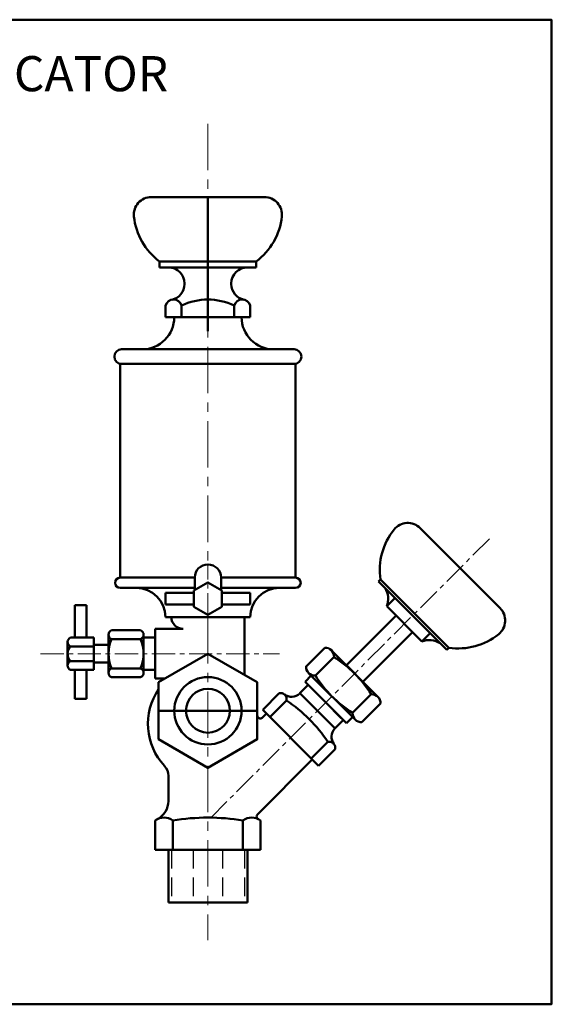
# Model space of a CAD drawing. Units: millimetres. Extents: x -414 to 17, y 81 to 417.
# Tile 7 of 7: x -165 to 17, y 81 to 417. Entities that reach past the tile are written whole.
import ezdxf

# ---------------------------------------------------------------- set-up
doc = ezdxf.new("R2010")
doc.units = ezdxf.units.MM
doc.header["$LTSCALE"] = 0.5
doc.linetypes.add('CENTER', pattern=[50.8, 31.75, -6.35, 6.35, -6.35])
doc.linetypes.add('DASHED', pattern=[19.05, 12.7, -6.35])
for name, color, linetype, lineweight in [('M-CNTR', 1, 'CENTER', 18), ('M-HIDN', 6, 'DASHED', 25), ('M-OUTL', 7, 'Continuous', 50), ('M-TEXT', 3, 'Continuous', 25)]:
    doc.layers.add(name, color=color, linetype=linetype, lineweight=lineweight)
doc.styles.get("Standard").update_dxf_attribs({"font": 'arial.ttf'})

msp = doc.modelspace()

# ---------------------------------------------------------------- linework, layer by layer
at = {"layer": 'M-CNTR'}
for p, q in [((-100.6, 381.5), (-100.6, 230.96)), ((-100.6, 212.96), (-100.6, 102.53))]:
    msp.add_line(p, q, dxfattribs=at)
at = {"layer": 'M-CNTR', "ltscale": 0.5}
for p, q in [((-4.33, 239.73), (-100.6, 143.46)), ((-100.6, 200.46), (-100.6, 230.96)), ((-157.84, 200.46), (-76.1, 200.46))]:
    msp.add_line(p, q, dxfattribs=at)
at = {"layer": 'M-HIDN'}
for p, q in [((-113.1, 133.46), (-113.1, 115.46)), ((-105.6, 133.46), (-105.6, 115.46)), ((-95.6, 133.46), (-95.6, 115.46)), ((-88.1, 133.46), (-88.1, 115.46))]:
    msp.add_line(p, q, dxfattribs=at)
at = {"layer": 'M-OUTL', "ltscale": 0.5}
for p, q in [((-119.94, 356.47), (-81.27, 356.47)), ((-100.6, 356.47), (-100.6, 334.47)), ((-117.1, 334.47), (-84.1, 334.47)), ((-117.1, 332.47), (-117.1, 334.47)), ((-84.1, 332.47), (-84.1, 334.47)), ((-117.1, 332.47), (-84.1, 332.47)), ((-28.01, 243.4), (-0.66, 216.06)), ((-105.1, 226.46), (-105.1, 222.18)), ((-96.1, 226.46), (-96.1, 222.18)), ((-42.27, 225.13), (-41.56, 225.84)), ((-41.56, 225.84), (-18.22, 202.5)), ((-42.27, 225.13), (-18.93, 201.8)), ((-42.27, 225.13), (-18.93, 201.8)), ((-105.37, 221.28), (-115.1, 221.28)), ((-115.1, 221.28), (-115.1, 217.28)), ((-95.84, 221.28), (-86.1, 221.28)), ((-86.1, 221.28), (-86.1, 217.28)), ((-39.44, 216.65), (-36.61, 219.48)), ((-146.1, 217.08), (-146.1, 205.96)), ((-146.1, 217.08), (-142.1, 217.08)), ((-142.1, 217.08), (-142.1, 205.96)), ((-105.37, 217.28), (-115.1, 217.28)), ((-95.84, 217.28), (-86.1, 217.28)), ((-39.44, 216.65), (-27.42, 204.63)), ((-115.1, 212.96), (-86.1, 212.96)), ((-115.1, 212.96), (-115.1, 212.96)), ((-88.1, 193.24), (-88.1, 212.96)), ((-86.1, 212.96), (-86.1, 212.96)), ((-53.23, 196.49), (-36.26, 213.46)), ((-36.26, 213.46), (-30.6, 207.81)), ((-118.6, 191.96), (-118.6, 208.96)), ((-118.6, 208.96), (-109.1, 208.96)), ((-147.6, 205.96), (-139.6, 205.96)), ((-139.6, 194.96), (-139.6, 205.96)), ((-134.6, 193.96), (-134.6, 206.96)), ((-133.6, 208.46), (-123.6, 208.46)), ((-133.6, 205.46), (-123.6, 205.46)), ((-122.6, 206.96), (-122.6, 193.96)), ((-122.6, 194.96), (-122.6, 205.96)), ((-122.6, 205.96), (-118.6, 205.96)), ((-30.6, 207.81), (-47.57, 190.84)), ((-24.59, 207.45), (-27.42, 204.63)), ((-148.6, 196.46), (-148.6, 204.46)), ((-147.6, 202.96), (-139.6, 202.96)), ((-139.6, 197.46), (-139.6, 203.46)), ((-139.6, 203.46), (-134.6, 203.46)), ((-134.6, 197.46), (-134.6, 203.46)), ((-134.6, 197.96), (-134.6, 202.96)), ((-67.01, 196.14), (-60.65, 202.5)), ((-18.22, 202.5), (-18.93, 201.8)), ((-63.83, 192.96), (-57.47, 199.32)), ((-58.41, 201.68), (-42.43, 185.7)), ((-147.6, 197.96), (-139.6, 197.96)), ((-139.6, 197.46), (-134.6, 197.46)), ((-133.6, 195.46), (-123.6, 195.46)), ((-47.57, 190.84), (-53.23, 196.49)), ((-147.6, 194.96), (-139.6, 194.96)), ((-146.1, 194.96), (-146.1, 185.08)), ((-142.1, 194.96), (-142.1, 185.08)), ((-123.6, 192.46), (-133.6, 192.46)), ((-122.6, 194.96), (-118.6, 194.96)), ((-118.6, 191.96), (-115.32, 191.96)), ((-67.37, 190.84), (-65.25, 192.96)), ((-50.12, 177.83), (-66.14, 193.85)), ((-69.17, 186.92), (-66.31, 189.78)), ((-53.23, 176.7), (-67.37, 190.84)), ((-146.1, 185.08), (-142.1, 185.08)), ((-76.21, 186.95), (-81.86, 181.29)), ((-74.22, 186.38), (-74.19, 186.4)), ((-69.14, 186.95), (-57.12, 174.93)), ((-44.74, 186.59), (-51.1, 180.23)), ((-73.73, 184.47), (-79.39, 178.82)), ((-60.3, 183.77), (-54.99, 178.46)), ((-41.56, 183.41), (-47.92, 177.05)), ((-117.49, 180.96), (-83.71, 180.96)), ((-82.01, 178.59), (-80.58, 180.01)), ((-81.86, 181.29), (-62.77, 162.2)), ((-53.23, 176.7), (-51.1, 178.82)), ((-57.15, 174.89), (-54.29, 177.76)), ((-65.25, 164.67), (-59.59, 170.33)), ((-62.77, 162.2), (-57.12, 167.86)), ((-83.66, 145.55), (-64.89, 164.32)), ((-118.6, 133.46), (-82.6, 133.46)), ((-114.1, 115.46), (-87.1, 115.46))]:
    msp.add_line(p, q, dxfattribs=at)
at = {"layer": 'M-OUTL'}
for p, q in [((-100.6, 310.61), (-100.6, 339.44)), ((-84.1, 332.47), (-100.6, 332.47)), ((-108.6, 326.78), (-108.6, 326.97)), ((-92.6, 326.78), (-92.6, 326.97)), ((-115.1, 319.46), (-115.1, 315.46)), ((-109.6, 319.46), (-109.6, 315.46)), ((-91.6, 319.46), (-91.6, 315.46)), ((-86.1, 315.46), (-86.1, 319.46)), ((-115.1, 315.46), (-86.1, 315.46)), ((-112.1, 315.46), (-89.1, 315.46)), ((-100.6, 315.46), (-100.6, 310.61)), ((-130.1, 304.46), (-78.1, 304.46)), ((-78.1, 304.46), (-71.1, 304.46)), ((-132.6, 301.96), (-132.6, 301.96)), ((-130.6, 299.46), (-130.6, 226.46)), ((-130.1, 299.46), (-71.1, 299.46)), ((-70.6, 299.46), (-70.6, 226.46)), ((-68.6, 301.96), (-68.6, 301.96)), ((-130.6, 226.46), (-105.1, 226.46)), ((-96.1, 226.46), (-70.6, 226.46)), ((-130.6, 222.96), (-105.1, 222.96)), ((-96.1, 222.96), (-70.6, 222.96)), ((-114.1, 158.68), (-114.1, 150.13)), ((-118.6, 143.46), (-118.6, 133.46)), ((-112.6, 143.46), (-112.6, 133.46)), ((-88.6, 143.46), (-88.6, 133.46)), ((-82.6, 143.46), (-82.6, 133.46)), ((-114.1, 133.46), (-114.1, 115.46)), ((-87.1, 133.46), (-87.1, 115.46))]:
    msp.add_line(p, q, dxfattribs=at)
at = {"layer": 'M-OUTL', "ltscale": 0.5}
for points in [[(-414.36, 417.09), (16.87, 417.09), (16.87, 80.66), (-414.36, 80.66)], [(-105.37, 222.03), (-105.37, 216.53), (-100.6, 213.78), (-95.84, 216.53), (-95.84, 222.03), (-100.6, 224.78)], [(-100.6, 161.46), (-83.71, 171.21), (-83.71, 190.71), (-100.6, 200.46), (-117.49, 190.71), (-117.49, 171.21)]]:
    msp.add_lwpolyline(points, close=True, dxfattribs=at)
for radius in [11.5, 7.5]:
    msp.add_circle((-100.6, 180.96), radius, dxfattribs=at)
for centre, radius, start, end in [((-119.94, 350.47), 6, 90, 186.0758), ((-81.27, 350.47), 6, 353.9242, 90), ((-104.03, 352.16), 22, 186.0758, 233.5379), ((-97.18, 352.16), 22, 306.4621, 353.9242), ((-19.8, 229.11), 22, 141.0758, 188.5379), ((-32.25, 239.16), 6, 45, 141.0758), ((-100.6, 226.46), 4.5, 0, 180), ((-130.6, 224.71), 1.75, 90, 270), ((-70.6, 224.71), 1.75, 270, 90), ((-45.96, 219.19), 7, 338.7269, 31.857), ((-4.91, 211.81), 6, 308.9242, 45), ((-109.1, 212.96), 4, 180, 270), ((-146.98, 204.46), 1.62, 112.6199, 247.3801), ((-132.98, 206.96), 1.63, 112.6199, 247.3801), ((-121.6, 200.46), 13, 157.3801, 202.6199), ((-124.23, 206.96), 1.62, 292.6199, 67.3801), ((-135.6, 200.46), 13, 337.3801, 22.6199), ((-14.96, 224.26), 22, 261.4621, 308.9242), ((-144.98, 200.46), 3.62, 136.3972, 223.6028), ((-60.49, 199.48), 3.03, 357.0244, 92.9756), ((-24.88, 198.1), 7, 58.143, 111.2731), ((-79.39, 164.67), 41, 32.3196, 57.6804), ((-146.98, 196.46), 1.63, 112.6199, 247.3801), ((-132.98, 193.96), 1.63, 112.6199, 247.3801), ((-124.23, 193.96), 1.62, 292.6199, 67.3801), ((-63.99, 195.99), 3.03, 177.0729, 272.9271), ((-29.18, 214.88), 41, 212.3196, 237.6804), ((-99.89, 176.52), 21.21, 146.0684, 222.865), ((-75.7, 184.98), 2.03, 345.5102, 104.4898), ((-72, 189.74), 4, 232.1434, 315), ((-44.59, 183.57), 3.03, 357.0731, 92.9269), ((-101.66, 142.4), 50.5, 33.5788, 56.4212), ((-82.71, 179.3), 1, 180, 315), ((-48.08, 180.07), 3.02, 176.9305, 273.0695), ((-54.32, 172.07), 4, 135, 217.8566), ((-59.08, 168.36), 2.03, 345.5102, 104.4898), ((-119.1, 158.68), 5, 0, 42.865), ((-121.1, 150.13), 7, 297.2796, 0), ((-82.95, 144.85), 1, 135, 243.8145), ((-115.6, 139.46), 5, 53.1301, 126.8699), ((-115.6, 139.46), 5, 117.2796, 126.8699), ((-100.6, 71.96), 72.5, 80.4727, 99.5273), ((-85.6, 139.46), 5, 53.1301, 126.8699), ((-81.72, 143.43), 0.879, 178.0179, 181.9821)]:
    msp.add_arc(centre, radius, start, end, dxfattribs=at)
at = {"layer": 'M-OUTL'}
for centre, radius, start, end in [((-114.1, 326.97), 5.5, 0, 90), ((-87.1, 326.97), 5.5, 90, 180), ((-114.1, 326.78), 5.5, 282.0389, 0), ((-87.1, 326.78), 5.5, 180, 257.9615), ((-112.35, 318.57), 2.89, 17.923, 162.077), ((-100.6, 300.21), 21.25, 64.9424, 115.0576), ((-88.85, 318.57), 2.89, 17.9401, 162.0599), ((-123.1, 315.46), 11, 270, 0), ((-78.1, 315.46), 11, 180, 270), ((-130.1, 301.96), 2.5, 90, 180), ((-71.1, 301.96), 2.5, 0, 90), ((-130.1, 301.96), 2.5, 180, 270), ((-71.1, 301.96), 2.5, 270, 0), ((-125.1, 212.96), 10, 0, 90), ((-76.1, 212.96), 10, 90, 180)]:
    msp.add_arc(centre, radius, start, end, dxfattribs=at)

# ---------------------------------------------------------------- texts
at = {"layer": 'M-TEXT', "ltscale": 0.5, "insert": (-337.22, 404.65), "char_height": 12, "attachment_point": 1}
msp.add_mtext_dynamic_manual_height_columns('\\pxqc;AUTOMATIC LUBRICATOR', width=250.9828, gutter_width=12.5, heights=[0], dxfattribs=at)

doc.saveas('drawing.dxf')
